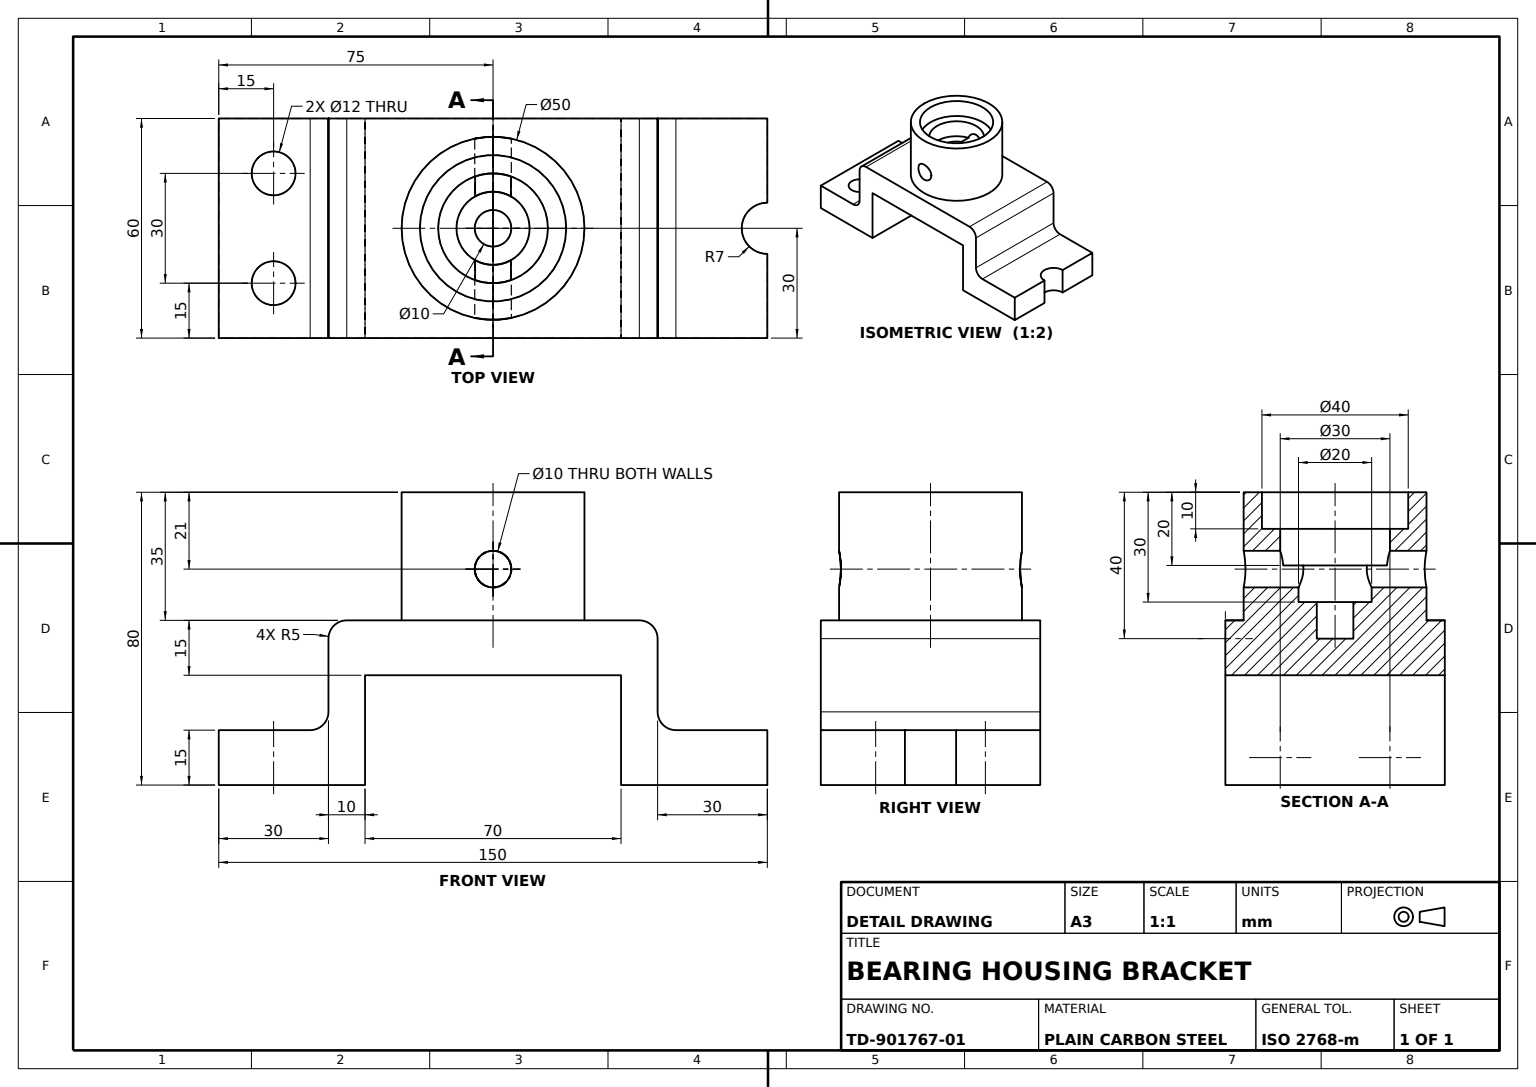
from build123d import *

# Parameters (mm, degrees)
BRACKET_BODY_DEPTH    = 30
FOOT_SLOT_A_REACH     = 88.168
FOOT_SLOT_A_SKETCH_R  = 6
FOOT_SLOT_B_REACH     = 88.168
BEARING_BOSS_SKETCH_R = 25
BEARING_BOSS_DEPTH    = 35
BORE_STEP_1_SKETCH_R  = 20
BORE_STEP_1_DEPTH     = 10
BORE_STEP_2_SKETCH_R  = 15
BORE_STEP_2_DEPTH     = 10
BORE_STEP_3_SKETCH_R  = 10
BORE_STEP_3_DEPTH     = 10
BORE_STEP_4_SKETCH_R  = 5
BORE_STEP_4_DEPTH     = 10
CROSS_HOLE_SKETCH_R   = 5
CROSS_HOLE_DEPTH      = 109.282039139
BEND_FILLET_R5_A_R    = 5
BEND_FILLET_R5_B_R    = 5
BEND_FILLET_R5_C_R    = 5


with BuildPart() as part:
    # Bracket Profile Sketch → Bracket Body (new, symmetric)
    with BuildSketch(Plane.XY):
        Polygon((-75, -30), (-35, -30), (-35, 0), (35, 0), (35, -30), (75, -30), (75, -15), (45, -15), (45, 15), (-45, 15), (-45, -15), (-75, -15), align=None)
    extrude(amount=BRACKET_BODY_DEPTH, both=True)

    # Foot Slot A Sketch → Foot Slot A (cut, up to next)
    with BuildSketch(Plane(origin=(0, -15, 0), x_dir=(1, 0, 0), z_dir=(0, 1, 0)), mode=Mode.PRIVATE) as foot_slot_a_sk1:
        with Locations(Location((-60, 15, 0), (0, 0, 180))):
            Circle(FOOT_SLOT_A_SKETCH_R)
    foot_slot_a_tool1 = extrude(foot_slot_a_sk1.sketch, amount=-FOOT_SLOT_A_REACH, mode=Mode.PRIVATE) & part.part
    # Foot Slot A Sketch → Foot Slot A (cut, up to next)
    with BuildSketch(Plane(origin=(0, -15, 0), x_dir=(1, 0, 0), z_dir=(0, 1, 0)), mode=Mode.PRIVATE) as foot_slot_a_sk2:
        with Locations(Location((-60, -15, 0), (0, 0, 180))):
            Circle(FOOT_SLOT_A_SKETCH_R)
    foot_slot_a_tool2 = extrude(foot_slot_a_sk2.sketch, amount=-FOOT_SLOT_A_REACH, mode=Mode.PRIVATE) & part.part
    add(foot_slot_a_tool1.solids().sort_by_distance((-60, -15, -15))[0], mode=Mode.SUBTRACT)
    add(foot_slot_a_tool2.solids().sort_by_distance((-60, -15, 15))[0], mode=Mode.SUBTRACT)

    # Foot Slot B Sketch → Foot Slot B (cut, up to next)
    with BuildSketch(Plane(origin=(0, -15, 0), x_dir=(1, 0, 0), z_dir=(0, 1, 0)), mode=Mode.PRIVATE) as foot_slot_b_sk1:
        with BuildLine():
            Line((75, 7), (75, -7))
            ThreePointArc((75, -7), (68, 0), (75, 7))
        make_face()
    foot_slot_b_tool1 = extrude(foot_slot_b_sk1.sketch, amount=-FOOT_SLOT_B_REACH, mode=Mode.PRIVATE) & part.part
    add(foot_slot_b_tool1.solids().sort_by_distance((72.029108, -15, 0))[0], mode=Mode.SUBTRACT)

    # Bearing Boss Sketch → Bearing Boss (add)
    with BuildSketch(Plane(origin=(0, 15, 0), x_dir=(1, 0, 0), z_dir=(0, 1, 0))):
        with Locations(Location((0, 0, 0), (0, 0, 180))):
            Circle(BEARING_BOSS_SKETCH_R)
    extrude(amount=BEARING_BOSS_DEPTH)

    # Bore Step 1 Sketch → Bore Step 1 (cut)
    with BuildSketch(Plane(origin=(0, 50, 0), x_dir=(1, 0, 0), z_dir=(0, 1, 0))):
        with Locations(Location((0, 0, 0), (0, 0, 180))):
            Circle(BORE_STEP_1_SKETCH_R)
    extrude(amount=-BORE_STEP_1_DEPTH, mode=Mode.SUBTRACT)

    # Bore Step 2 Sketch → Bore Step 2 (cut)
    with BuildSketch(Plane(origin=(0, 40, 0), x_dir=(1, 0, 0), z_dir=(0, 1, 0))):
        with Locations(Location((0, 0, 0), (0, 0, 180))):
            Circle(BORE_STEP_2_SKETCH_R)
    extrude(amount=-BORE_STEP_2_DEPTH, mode=Mode.SUBTRACT)

    # Bore Step 3 Sketch → Bore Step 3 (cut)
    with BuildSketch(Plane(origin=(0, 30, 0), x_dir=(1, 0, 0), z_dir=(0, 1, 0))):
        with Locations(Location((0, 0, 0), (0, 0, 180))):
            Circle(BORE_STEP_3_SKETCH_R)
    extrude(amount=-BORE_STEP_3_DEPTH, mode=Mode.SUBTRACT)

    # Bore Step 4 Sketch → Bore Step 4 (cut)
    with BuildSketch(Plane(origin=(0, 20, 0), x_dir=(1, 0, 0), z_dir=(0, 1, 0))):
        with Locations(Location((0, 0, 0), (0, 0, 180))):
            Circle(BORE_STEP_4_SKETCH_R)
    extrude(amount=-BORE_STEP_4_DEPTH, mode=Mode.SUBTRACT)

    # Cross Hole Sketch → Cross Hole (cut, through all)
    with BuildSketch(Plane.XY.offset(30)):
        with Locations((0, 29)):
            Circle(CROSS_HOLE_SKETCH_R)
    extrude(amount=-CROSS_HOLE_DEPTH, mode=Mode.SUBTRACT)

    # Bend Fillet R5 A
    bend_fillet_r5_a_edges = [part.edges().sort_by_distance(p)[0] for p in [
        (45, -15, 0),
    ]]
    fillet(bend_fillet_r5_a_edges, radius=BEND_FILLET_R5_A_R)

    # Bend Fillet R5 B
    bend_fillet_r5_b_edges = [part.edges().sort_by_distance(p)[0] for p in [
        (-45, 15, 0),
        (45, 15, 0),
    ]]
    fillet(bend_fillet_r5_b_edges, radius=BEND_FILLET_R5_B_R)

    # Bend Fillet R5 C
    bend_fillet_r5_c_edges = [part.edges().sort_by_distance(p)[0] for p in [
        (-45, -15, 0),
    ]]
    fillet(bend_fillet_r5_c_edges, radius=BEND_FILLET_R5_C_R)


solid = part.part
